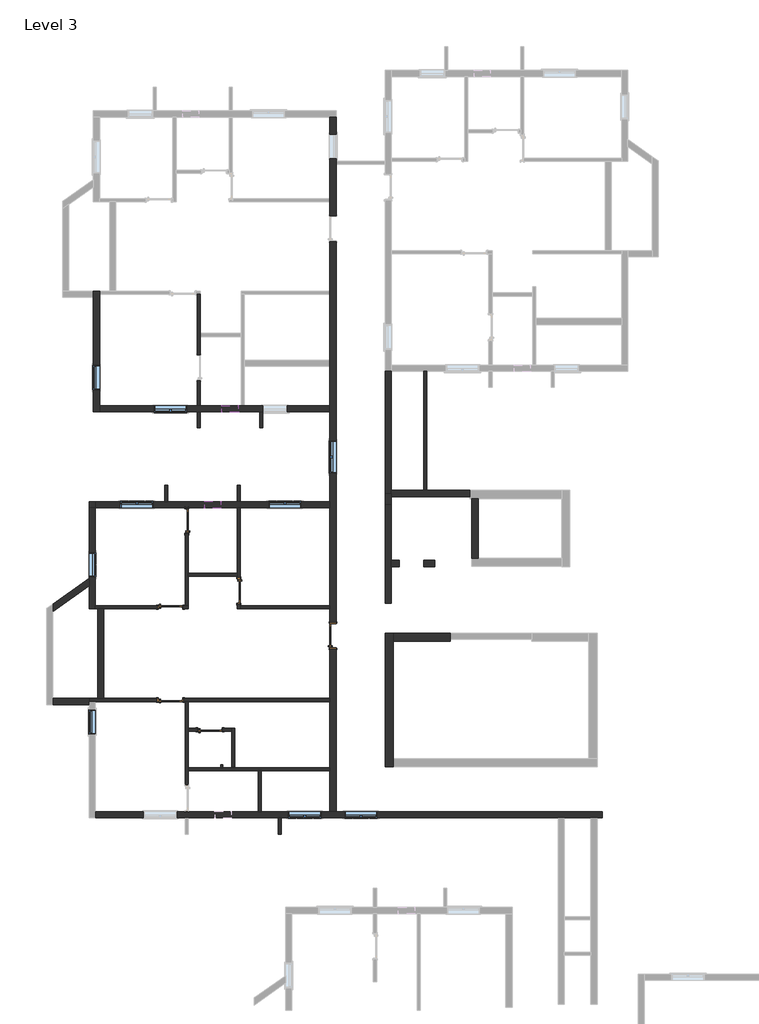
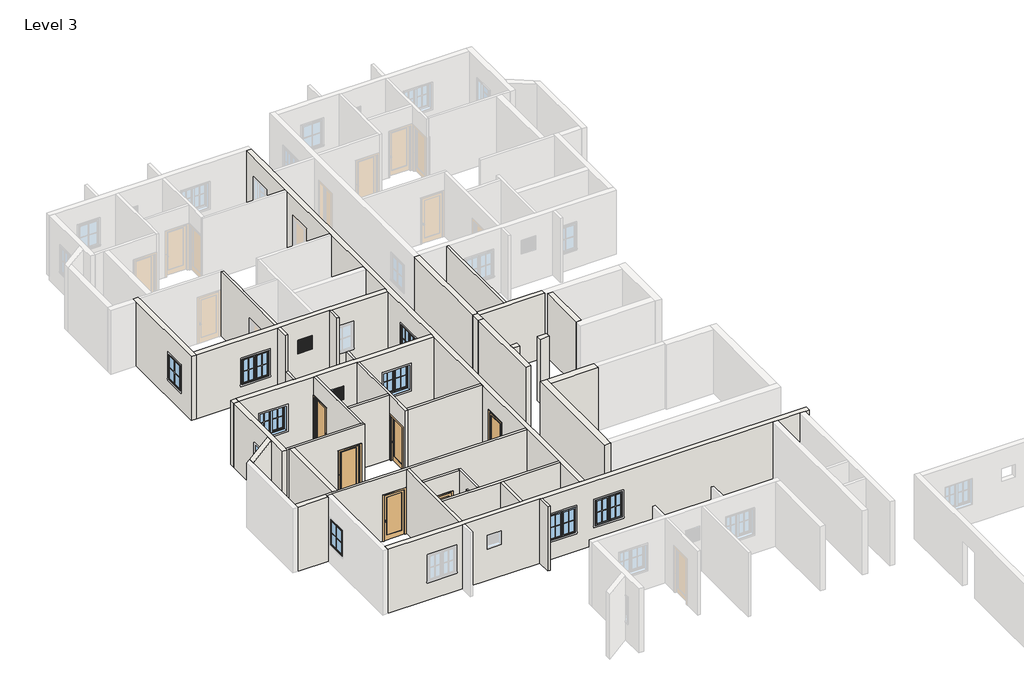
# One storey, part 4 of 7: 38 walls, 11 windows, 6 doors.
# Revit data of these elements (continued)
# Element 46 (IfcWindow, "Window-Awning-Single : 36\" x 48\"") (continued)
#   Mark = "21"
#   Window Inset = 0' - 0"
#   Interior Wall Closure = 0' - 2 1/4"
#   Frame Extension = 0' - 0 1/4"
#   Exterior Wall Closure = 0' - 1 1/4"
#   Interior Trim Visibility = yes
#   Exterior Trim Visibility = yes
#   Phase Created = New Construction
#   Materials on its faces: "Wood - Stained", "Glass", "Clad - White"
# Element 47 (IfcWindow, "Window-Awning-Single : 36\" x 48\"")
#   Mark = "33"
#   Window Inset = 0' - 0"
#   Interior Wall Closure = 0' - 2 1/4"
#   Frame Extension = 0' - 0 1/4"
#   Exterior Wall Closure = 0' - 1 1/4"
#   Interior Trim Visibility = yes
#   Exterior Trim Visibility = yes
#   Phase Created = New Construction
#   Materials on its faces: "Wood - Stained", "Glass", "Clad - White"
# Element 48 (IfcWindow, "Window-Casement-Double : 4' x 4'")
#   Mark = "36"
#   Window Inset = 0' - 0"
#   Interior Wall Closure = 0' - 2 1/4"
#   Frame Extension = 0' - 0 1/4"
#   Exterior Wall Closure = 0' - 1 1/4"
#   Interior Trim Visibility = yes
#   Exterior Trim Visibility = yes
#   Phase Created = New Construction
#   Materials on its faces: "Wood - Stained", "Glass", "Clad - White"
# Element 49 (IfcWindow, "Window-Casement-Double : 4' x 4'")
#   Mark = "61"
#   Window Inset = 0' - 0"
#   Interior Wall Closure = 0' - 2 1/4"
#   Frame Extension = 0' - 0 1/4"
#   Exterior Wall Closure = 0' - 1 1/4"
#   Interior Trim Visibility = yes
#   Exterior Trim Visibility = yes
#   Phase Created = New Construction
#   Materials on its faces: "Wood - Stained", "Glass", "Clad - White"
# Element 50 (IfcWindow, "Window-Casement-Double : 4' x 4'")
#   Mark = "62"
#   Window Inset = 0' - 0"
#   Interior Wall Closure = 0' - 2 1/4"
#   Frame Extension = 0' - 0 1/4"
#   Exterior Wall Closure = 0' - 1 1/4"
#   Interior Trim Visibility = yes
#   Exterior Trim Visibility = yes
#   Phase Created = New Construction
#   Materials on its faces: "Wood - Stained", "Glass", "Clad - White"
# Element 51 (IfcWindow, "Window-Casement-Double : 4' x 4'")
#   Mark = "64"
#   Window Inset = 0' - 0"
#   Interior Wall Closure = 0' - 2 1/4"
#   Frame Extension = 0' - 0 1/4"
#   Exterior Wall Closure = 0' - 1 1/4"
#   Interior Trim Visibility = yes
#   Exterior Trim Visibility = yes
#   Phase Created = New Construction
#   Materials on its faces: "Wood - Stained", "Glass", "Clad - White"
# Element 52 (IfcWindow, "Window-Casement-Double : 4' x 4'")
#   Mark = "65"
#   Window Inset = 0' - 0"
#   Interior Wall Closure = 0' - 2 1/4"
#   Frame Extension = 0' - 0 1/4"
#   Exterior Wall Closure = 0' - 1 1/4"
#   Interior Trim Visibility = yes
#   Exterior Trim Visibility = yes
#   Phase Created = New Construction
#   Materials on its faces: "Wood - Stained", "Glass", "Clad - White"
# Element 53 (IfcWindow, "Window-Casement-Double : 4' x 4'")
#   Mark = "66"
#   Window Inset = 0' - 0"
#   Interior Wall Closure = 0' - 2 1/4"
#   Frame Extension = 0' - 0 1/4"
#   Exterior Wall Closure = 0' - 1 1/4"
#   Interior Trim Visibility = yes
#   Exterior Trim Visibility = yes
#   Phase Created = New Construction
#   Materials on its faces: "Wood - Stained", "Glass", "Clad - White"
# Element 54 (IfcWindow, "Window-Louvers : 24\" x 24\"")
#   Mark = "2"
#   Blade Width = 1' - 10 1/2"
#   Phase Created = New Construction
#   Materials on its faces: "Birch"
# Element 55 (IfcWindow, "Window-Louvers : 24\" x 24\"")
#   Mark = "5"
#   Blade Width = 1' - 10 1/2"
#   Phase Created = New Construction
#   Materials on its faces: "Birch"
# Materials
#   "Cherry": class "Wood", colour RGB 226 177 128, transparency 0, Description = "Prunus Serotina", Cost = 0
#   "Aluminum": class "Metal", colour RGB 247 247 247, transparency 0, Description = "Aluminum 6061", Cost = 0
#   "Wood - Stained": class "Wood", colour RGB 224 178 126, transparency 0, Cost = 0
#   "Glass": class "Glass", colour RGB 0 128 192, transparency 0.75, Description = "Soda Lime Glass", Cost = 0
#   "Clad - White": class "Wood", colour RGB 242 242 238, transparency 0, Cost = 0
#   "Birch": class "Wood", colour RGB 224 178 126, transparency 0, Description = "Betula Alleghaniensis", Cost = 0
#   "Default Wall": colour RGB 128 128 128, transparency 0, Cost = 0
